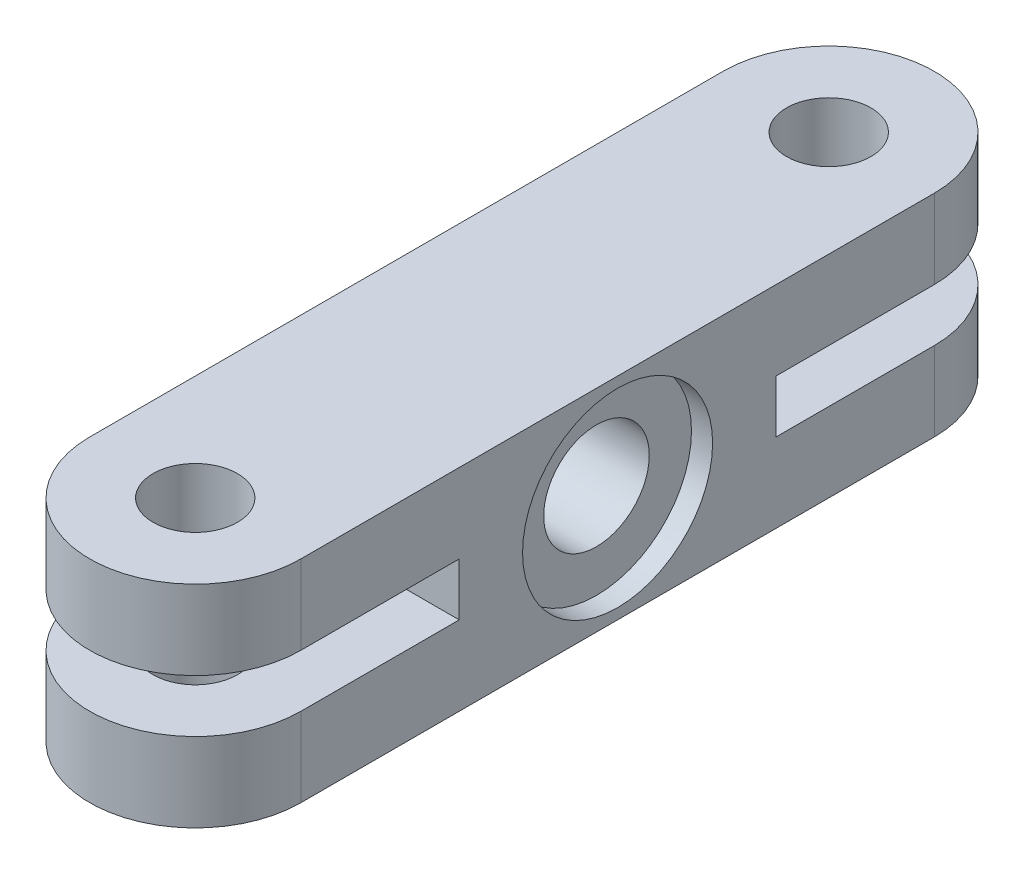
SolidWorks part; units mm, degrees
material "Plain Carbon Steel"
ref_plane "Front Plane" through (0, 0, 0) normal (0, 0, 1) x (1, 0, 0)
ref_plane "Top Plane" through (0, 0, 0) normal (0, 1, 0) x (1, 0, 0)
ref_plane "Right Plane" through (0, 0, 0) normal (1, 0, 0) x (0, 0, -1)
sketch "Link Body Sketch" plane through (0, 0, 0) normal (0, 1, 0) x (1, 0, 0)
  line L0 (-617.3424, 0) -> (30249.7763, 0) construction
  line L1 (0, -617.3424) -> (0, 30249.7763) construction
  line L2 (0, 30) -> (0, -30) construction
  line L3 (10, 30) -> (10, -30)
  line L4 (-10, 30) -> (-10, -30)
  arc A0 (10, 30) -> (-10, 30) centre (0, 30) ccw
  arc A1 (-10, -30) -> (10, -30) centre (0, -30) ccw
  point P7 (0, 0)
  dimension "D1" = 10
  dimension "D2" = 60
  dimension "D3" = 30
extrude "Link Body" add sketch "Link Body Sketch" along normal mid plane 20
sketch "Pin Holes Sketch" plane through (0, 0, 0) normal (0, 1, 0) x (1, 0, 0)
  circle A0 centre (0, 30) radius 4
  circle A1 centre (0, -30) radius 4
  dimension "D1" = 8
  dimension "D2" = 8
extrude "Pin Holes 2xØ8" cut sketch "Pin Holes Sketch" against normal mid plane 20
sketch "Side Slots Sketch" plane through (0, 0, 0) normal (1, 0, 0) x (0, 0, -1)
  line L0 (-1000, 0) -> (49000, 0) construction
  line L1 (0, -1000) -> (0, 49000) construction
  line L2 (40, -10) -> (40, 10) construction
  line L3 (-45.7528, 2.5) -> (-15, 2.5)
  line L4 (-45.7528, 2.5) -> (-45.7528, -2.5)
  line L5 (-45.7528, -2.5) -> (-15, -2.5)
  line L6 (-15, 2.5) -> (-15, -2.5)
  line L7 (15, 2.5) -> (44.5374, 2.5)
  line L8 (15, 2.5) -> (15, -2.5)
  line L9 (15, -2.5) -> (44.5374, -2.5)
  line L10 (44.5374, 2.5) -> (44.5374, -2.5)
  line L11 (-40, 10) -> (-40, -10) construction
  circle A0 centre (0, 0) radius 5
  dimension "D9" = 10
  dimension "D1" = 5
  dimension "D2" = 2.5
  dimension "D3" = 5
  dimension "D4" = 2.5
  dimension "D5" = 25
  dimension "D6" = 25
  dimension "D7" = 30.7528
  dimension "D8" = 29.5374
extrude "Side Slots Cut" cut sketch "Side Slots Sketch" against normal mid plane 20
sketch "Counterbore Sketch" plane through (10, 0, 0) normal (1, 0, 0) x (0, 0, -1)
  circle A0 centre (0, 0) radius 9
  dimension "D1" = 18
extrude "Counterbore Ø18x2" cut sketch "Counterbore Sketch" against normal blind 2
